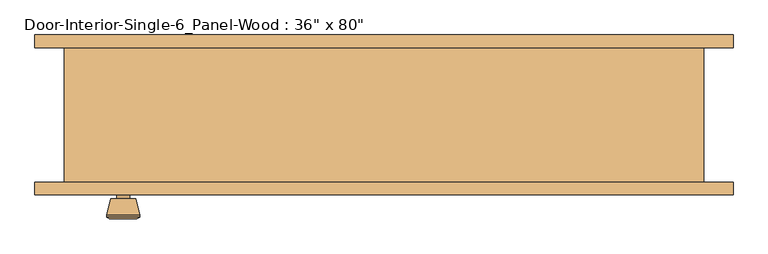
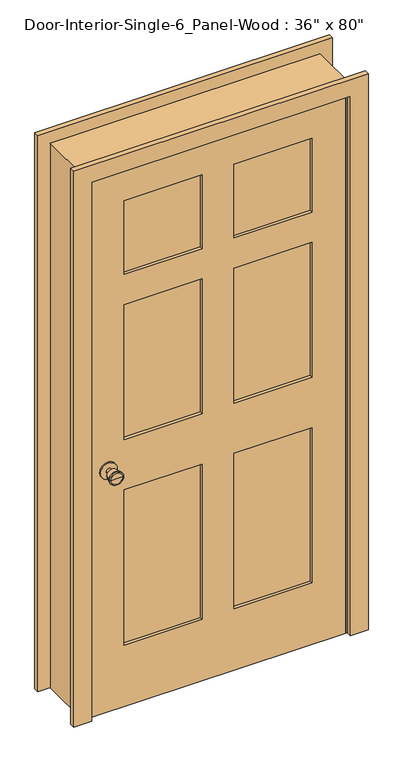
"""IFC4 building model written with IfcOpenShell, lengths in millimetres: door geometry."""

from ifc_helpers import new_model, si_unit, point, frame, frame_2d, origin, place, context, project, spatial, polyline, circle_curve, trimmed, segment, composite_curve, outline, extrude, faceted_brep, source, transform, mapped, element, save
from ifc_brep_helpers import plane_surface, cylinder_surface, revolved_surface, advanced_brep


def door_c2afa946(model_context):
    return source(origin(), model_context, "Body", "SolidModel", [
        advanced_brep(
        [(-393.7, -57.5, 914.4), (-403.7, -57.5, 914.4), (-383.7, -57.5, 914.4), (-373.2241324, -8.5, 914.4), (-414.1758676, -8.5, 914.4), (-393.7, -8.5, 914.4), (-368.7, -10.3278681, 914.4), (-418.7, -10.3278681, 914.4), (-368.7, -13.7915463, 914.4), (-418.7, -13.7915463, 914.4), (-375.063764, -38.5, 914.4), (-412.336236, -38.5, 914.4), (-383.7, -38.5, 914.4), (-403.7, -38.5, 914.4)],
        [
            (0, 1),
            (1, 2, circle_curve(frame((-393.7, -57.5, 914.4), z_axis=(0.0, -1.0, 0.0), x_axis=(-1.0, 0.0, 0.0)), 10.0)),
            (2, 0),
            (2, 1, circle_curve(frame((-393.7, -57.5, 914.4), z_axis=(0.0, -1.0, 0.0), x_axis=(-1.0, 0.0, 0.0)), 10.0)),
            (3, 4, circle_curve(frame((-393.7, -8.5, 914.4), z_axis=(0.0, 1.0, 0.0), x_axis=(-1.0, 0.0, 0.0)), 20.4758676)),
            (4, 5),
            (5, 3),
            (4, 3, circle_curve(frame((-393.7, -8.5, 914.4), z_axis=(0.0, 1.0, 0.0), x_axis=(-1.0, 0.0, 0.0)), 20.4758676)),
            (6, 7, circle_curve(frame((-393.7, -10.3278681, 914.4), z_axis=(0.0, 1.0, 0.0), x_axis=(-1.0, 0.0, 0.0)), 25.0)),
            (7, 4),
            (3, 6),
            (7, 6, circle_curve(frame((-393.7, -10.3278681, 914.4), z_axis=(0.0, 1.0, 0.0), x_axis=(-1.0, 0.0, 0.0)), 25.0)),
            (8, 9, circle_curve(frame((-393.7, -13.7915463, 914.4), z_axis=(0.0, 1.0, 0.0), x_axis=(-1.0, 0.0, 0.0)), 25.0)),
            (9, 7),
            (6, 8),
            (9, 8, circle_curve(frame((-393.7, -13.7915463, 914.4), z_axis=(0.0, 1.0, 0.0), x_axis=(-1.0, 0.0, 0.0)), 25.0)),
            (10, 11, circle_curve(frame((-393.7, -38.5, 914.4), z_axis=(0.0, 1.0, 0.0), x_axis=(-1.0, 0.0, 0.0)), 18.636236)),
            (11, 9),
            (8, 10),
            (11, 10, circle_curve(frame((-393.7, -38.5, 914.4), z_axis=(0.0, 1.0, 0.0), x_axis=(-1.0, 0.0, 0.0)), 18.636236)),
            (12, 13, circle_curve(frame((-393.7, -38.5, 914.4), z_axis=(0.0, 1.0, 0.0), x_axis=(-1.0, 0.0, 0.0)), 10.0)),
            (13, 11),
            (10, 12),
            (13, 12, circle_curve(frame((-393.7, -38.5, 914.4), z_axis=(0.0, 1.0, 0.0), x_axis=(-1.0, 0.0, 0.0)), 10.0)),
            (1, 13),
            (12, 2),
        ],
        [
            plane_surface(frame((-393.7, -57.5, 914.4), z_axis=(0.0, -1.0, 0.0), x_axis=(-1.0, 0.0, 0.0))),
            plane_surface(frame((-393.7, -8.5, 914.4), z_axis=(0.0, 1.0, 0.0), x_axis=(-1.0, 0.0, 0.0))),
            revolved_surface(polyline([(-414.1758676, -8.5, 914.4), (-418.7, -10.3278681, 914.4)]), (-393.7, -57.5, 914.4), (0.0, -1.0, 0.0)),
            cylinder_surface(frame((-393.7, -57.5, 914.4), z_axis=(0.0, -1.0, 0.0), x_axis=(-1.0, 0.0, 0.0)), 25.0),
            revolved_surface(polyline([(-418.7, -13.7915463, 914.4), (-412.336236, -38.5, 914.4)]), (-393.7, -57.5, 914.4), (0.0, -1.0, 0.0)),
            plane_surface(frame((-393.7, -38.5, 914.4), z_axis=(0.0, -1.0, 0.0), x_axis=(-1.0, 0.0, 0.0))),
            cylinder_surface(frame((-393.7, -57.5, 914.4), z_axis=(0.0, -1.0, 0.0), x_axis=(-1.0, 0.0, 0.0)), 10.0),
        ],
        [
            (0, [[1, 2, 3]]),
            (0, [[-3, 4, -1]]),
            (1, [[5, 6, 7]]),
            (1, [[8, -7, -6]]),
            (2, [[9, 10, -5, 11]]),
            (2, [[12, -11, -8, -10]]),
            (3, [[13, 14, -9, 15]]),
            (3, [[16, -15, -12, -14]]),
            (4, [[17, 18, -13, 19]]),
            (4, [[20, -19, -16, -18]]),
            (5, [[21, 22, -17, 23]]),
            (5, [[24, -23, -20, -22]]),
            (6, [[-2, 25, -21, 26]]),
            (6, [[-4, -26, -24, -25]]),
        ],
    ),
        extrude(outline(composite_curve([segment(trimmed(circle_curve(frame_2d((914.4, -393.7)), 30.0), [point((914.4, -423.7))], [point((914.4, -363.7))], False, "CARTESIAN"), True, "CONTINUOUS"), segment(trimmed(circle_curve(frame_2d((914.4, -393.7)), 30.0), [point((914.4, -363.7))], [point((914.4, -423.7))], False, "CARTESIAN"), True, "CONTINUOUS")], self_intersect=False)), frame((0.0, -63.5, 0.0), z_axis=(0.0, 1.0, 0.0), x_axis=(0.0, 0.0, 1.0)), (0.0, 0.0, 1.0), 6.0),
        advanced_brep(
        [(-393.7, -104.425, 914.4), (-383.7, -104.425, 914.4), (-403.7, -104.425, 914.4), (-373.2241324, -153.425, 914.4), (-393.7, -153.425, 914.4), (-414.1758676, -153.425, 914.4), (-368.7, -151.5971319, 914.4), (-418.7, -151.5971319, 914.4), (-368.7, -148.1334537, 914.4), (-418.7, -148.1334537, 914.4), (-375.063764, -123.425, 914.4), (-412.336236, -123.425, 914.4), (-383.7, -123.425, 914.4), (-403.7, -123.425, 914.4)],
        [
            (0, 1),
            (1, 2, circle_curve(frame((-393.7, -104.425, 914.4), z_axis=(0.0, 1.0, 0.0), x_axis=(-1.0, 0.0, 0.0)), 10.0)),
            (2, 0),
            (2, 1, circle_curve(frame((-393.7, -104.425, 914.4), z_axis=(0.0, 1.0, 0.0), x_axis=(-1.0, 0.0, 0.0)), 10.0)),
            (3, 4),
            (4, 5),
            (5, 3, circle_curve(frame((-393.7, -153.425, 914.4), z_axis=(0.0, -1.0, 0.0), x_axis=(-1.0, 0.0, 0.0)), 20.4758676)),
            (3, 5, circle_curve(frame((-393.7, -153.425, 914.4), z_axis=(0.0, -1.0, 0.0), x_axis=(-1.0, 0.0, 0.0)), 20.4758676)),
            (6, 3),
            (5, 7),
            (7, 6, circle_curve(frame((-393.7, -151.5971319, 914.4), z_axis=(0.0, -1.0, 0.0), x_axis=(-1.0, 0.0, 0.0)), 25.0)),
            (6, 7, circle_curve(frame((-393.7, -151.5971319, 914.4), z_axis=(0.0, -1.0, 0.0), x_axis=(-1.0, 0.0, 0.0)), 25.0)),
            (8, 6),
            (7, 9),
            (9, 8, circle_curve(frame((-393.7, -148.1334537, 914.4), z_axis=(0.0, -1.0, 0.0), x_axis=(-1.0, 0.0, 0.0)), 25.0)),
            (8, 9, circle_curve(frame((-393.7, -148.1334537, 914.4), z_axis=(0.0, -1.0, 0.0), x_axis=(-1.0, 0.0, 0.0)), 25.0)),
            (10, 8),
            (9, 11),
            (11, 10, circle_curve(frame((-393.7, -123.425, 914.4), z_axis=(0.0, -1.0, 0.0), x_axis=(-1.0, 0.0, 0.0)), 18.636236)),
            (10, 11, circle_curve(frame((-393.7, -123.425, 914.4), z_axis=(0.0, -1.0, 0.0), x_axis=(-1.0, 0.0, 0.0)), 18.636236)),
            (12, 10),
            (11, 13),
            (13, 12, circle_curve(frame((-393.7, -123.425, 914.4), z_axis=(0.0, -1.0, 0.0), x_axis=(-1.0, 0.0, 0.0)), 10.0)),
            (12, 13, circle_curve(frame((-393.7, -123.425, 914.4), z_axis=(0.0, -1.0, 0.0), x_axis=(-1.0, 0.0, 0.0)), 10.0)),
            (1, 12),
            (13, 2),
        ],
        [
            plane_surface(frame((-393.7, -104.425, 914.4), z_axis=(0.0, 1.0, 0.0), x_axis=(-1.0, 0.0, 0.0))),
            plane_surface(frame((-393.7, -153.425, 914.4), z_axis=(0.0, -1.0, 0.0), x_axis=(-1.0, 0.0, 0.0))),
            revolved_surface(polyline([(-414.1758676, -153.425, 914.4), (-418.7, -151.5971319, 914.4)]), (-393.7, -104.425, 914.4), (0.0, 1.0, 0.0)),
            cylinder_surface(frame((-393.7, -104.425, 914.4), z_axis=(0.0, 1.0, 0.0), x_axis=(-1.0, 0.0, 0.0)), 25.0),
            revolved_surface(polyline([(-418.7, -148.1334537, 914.4), (-412.336236, -123.425, 914.4)]), (-393.7, -104.425, 914.4), (0.0, 1.0, 0.0)),
            plane_surface(frame((-393.7, -123.425, 914.4), z_axis=(0.0, 1.0, 0.0), x_axis=(-1.0, 0.0, 0.0))),
            cylinder_surface(frame((-393.7, -104.425, 914.4), z_axis=(0.0, 1.0, 0.0), x_axis=(-1.0, 0.0, 0.0)), 10.0),
        ],
        [
            (0, [[1, 2, 3]]),
            (0, [[-3, 4, -1]]),
            (1, [[5, 6, 7]]),
            (1, [[-6, -5, 8]]),
            (2, [[9, -7, 10, 11]]),
            (2, [[-10, -8, -9, 12]]),
            (3, [[13, -11, 14, 15]]),
            (3, [[-14, -12, -13, 16]]),
            (4, [[17, -15, 18, 19]]),
            (4, [[-18, -16, -17, 20]]),
            (5, [[21, -19, 22, 23]]),
            (5, [[-22, -20, -21, 24]]),
            (6, [[25, -23, 26, -2]]),
            (6, [[-26, -24, -25, -4]]),
        ],
    ),
        extrude(outline(composite_curve([segment(trimmed(circle_curve(frame_2d((914.4, -393.7)), 30.0), [point((914.4, -423.7))], [point((914.4, -363.7))], False, "CARTESIAN"), True, "CONTINUOUS"), segment(trimmed(circle_curve(frame_2d((914.4, -393.7)), 30.0), [point((914.4, -363.7))], [point((914.4, -423.7))], False, "CARTESIAN"), True, "CONTINUOUS")], self_intersect=False)), frame((0.0, -104.425, 0.0), z_axis=(0.0, 1.0, 0.0), x_axis=(0.0, 0.0, 1.0)), (0.0, 0.0, 1.0), 6.0),
        extrude(outline(polyline([(336.55, -75.1416667), (336.55, -86.7833333), (57.15, -86.7833333), (57.15, -75.1416667), (336.55, -75.1416667)])), frame((0.0, 0.0, 1633.5375), z_axis=(0.0, 0.0, 1.0), x_axis=(1.0, 0.0, 0.0)), (0.0, 0.0, 1.0), 279.4),
        extrude(outline(polyline([(336.55, -75.1416667), (336.55, -86.7833333), (57.15, -86.7833333), (57.15, -75.1416667), (336.55, -75.1416667)])), frame((0.0, 0.0, 1009.65), z_axis=(0.0, 0.0, 1.0), x_axis=(1.0, 0.0, 0.0)), (0.0, 0.0, 1.0), 509.5875),
        extrude(outline(polyline([(-57.15, -75.1416667), (-57.15, -86.7833333), (-336.55, -86.7833333), (-336.55, -75.1416667), (-57.15, -75.1416667)])), frame((0.0, 0.0, 1009.65), z_axis=(0.0, 0.0, 1.0), x_axis=(1.0, 0.0, 0.0)), (0.0, 0.0, 1.0), 509.5875),
        extrude(outline(polyline([(-57.15, -75.1416667), (-57.15, -86.7833333), (-336.55, -86.7833333), (-336.55, -75.1416667), (-57.15, -75.1416667)])), frame((0.0, 0.0, 1633.5375), z_axis=(0.0, 0.0, 1.0), x_axis=(1.0, 0.0, 0.0)), (0.0, 0.0, 1.0), 279.4),
        extrude(outline(polyline([(336.55, -75.1416667), (336.55, -86.7833333), (57.15, -86.7833333), (57.15, -75.1416667), (336.55, -75.1416667)])), frame((0.0, 0.0, 231.775), z_axis=(0.0, 0.0, 1.0), x_axis=(1.0, 0.0, 0.0)), (0.0, 0.0, 1.0), 587.375),
        extrude(outline(polyline([(-57.15, -75.1416667), (-57.15, -86.7833333), (-336.55, -86.7833333), (-336.55, -75.1416667), (-57.15, -75.1416667)])), frame((0.0, 0.0, 231.775), z_axis=(0.0, 0.0, 1.0), x_axis=(1.0, 0.0, 0.0)), (0.0, 0.0, 1.0), 587.375),
        extrude(outline(polyline([(2032.0, -457.2), (0.0, -457.2), (0.0, 457.2), (2032.0, 457.2), (2032.0, -457.2)]), holes=[polyline([(1912.9375, 57.15), (1912.9375, 336.55), (1633.5375, 336.55), (1633.5375, 57.15), (1912.9375, 57.15)]), polyline([(1519.2375, 336.55), (1009.65, 336.55), (1009.65, 57.15), (1519.2375, 57.15), (1519.2375, 336.55)]), polyline([(1009.65, -57.15), (1009.65, -336.55), (1519.2375, -336.55), (1519.2375, -57.15), (1009.65, -57.15)]), polyline([(1633.5375, -336.55), (1912.9375, -336.55), (1912.9375, -57.15), (1633.5375, -57.15), (1633.5375, -336.55)]), polyline([(819.15, 57.15), (819.15, 336.55), (231.775, 336.55), (231.775, 57.15), (819.15, 57.15)]), polyline([(231.775, -57.15), (231.775, -336.55), (819.15, -336.55), (819.15, -57.15), (231.775, -57.15)])]), frame((0.0, -98.425, 0.0), z_axis=(0.0, 1.0, 0.0), x_axis=(0.0, 0.0, 1.0)), (0.0, 0.0, 1.0), 34.925),
        faceted_brep([(482.6, -98.425, 0.0), (457.2, -98.425, 0.0), (457.2, -63.5, 0.0), (444.5, -63.5, 0.0), (444.5, -28.575, 0.0), (457.2, -28.575, 0.0), (457.2, 104.775, 0.0), (482.6, 104.775, 0.0), (482.6, 104.775, 2057.4), (482.6, -98.425, 2057.4), (457.2, 104.775, 2032.0), (-457.2, 104.775, 2032.0), (-457.2, 104.775, 0.0), (-482.6, 104.775, 0.0), (-482.6, 104.775, 2057.4), (457.2, -28.575, 2032.0), (444.5, -28.575, 2019.3), (-444.5, -28.575, 2019.3), (-444.5, -28.575, 0.0), (-457.2, -28.575, 0.0), (-457.2, -28.575, 2032.0), (444.5, -63.5, 2019.3), (457.2, -63.5, 2032.0), (-457.2, -63.5, 2032.0), (-457.2, -63.5, 0.0), (-444.5, -63.5, 0.0), (-444.5, -63.5, 2019.3), (457.2, -98.425, 2032.0), (-482.6, -98.425, 2057.4), (-482.6, -98.425, 0.0), (-457.2, -98.425, 0.0), (-457.2, -98.425, 2032.0)], [[[0, 1, 2, 3, 4, 5, 6, 7]], [[7, 8, 9, 0]], [[6, 10, 11, 12, 13, 14, 8, 7]], [[5, 15, 10, 6]], [[4, 16, 17, 18, 19, 20, 15, 5]], [[3, 21, 16, 4]], [[2, 22, 23, 24, 25, 26, 21, 3]], [[1, 27, 22, 2]], [[0, 9, 28, 29, 30, 31, 27, 1]], [[8, 14, 28, 9]], [[15, 20, 11, 10]], [[21, 26, 17, 16]], [[27, 31, 23, 22]], [[29, 13, 12, 19, 18, 25, 24, 30]], [[14, 13, 29, 28]], [[20, 19, 12, 11]], [[26, 25, 18, 17]], [[31, 30, 24, 23]]]),
        extrude(outline(polyline([(0.0, 527.05), (2101.85, 527.05), (2101.85, -527.05), (0.0, -527.05), (0.0, -463.55), (2038.35, -463.55), (2038.35, 463.55), (0.0, 463.55), (0.0, 527.05)])), frame((0.0, 104.775, 0.0), z_axis=(0.0, 1.0, 0.0), x_axis=(0.0, 0.0, 1.0)), (0.0, 0.0, 1.0), 19.05),
        extrude(outline(polyline([(0.0, 527.05), (2101.85, 527.05), (2101.85, -527.05), (0.0, -527.05), (0.0, -463.55), (2038.35, -463.55), (2038.35, 463.55), (0.0, 463.55), (0.0, 527.05)])), frame((0.0, -117.475, 0.0), z_axis=(0.0, 1.0, 0.0), x_axis=(0.0, 0.0, 1.0)), (0.0, 0.0, 1.0), 19.05),
    ])


if __name__ == "__main__":
    model = new_model("IFC4")
    model_context = context("Model", 3, world=origin())
    ifc_project = project(units=[si_unit("LENGTHUNIT", "METRE", prefix="MILLI")], contexts=[model_context])
    site = spatial("IfcSite", under=ifc_project)
    building = spatial("IfcBuilding", under=site)
    placement = place(None, origin())
    door_shape = door_c2afa946(model_context)
    element("IfcDoor", 1, ObjectType="Door-Interior-Single-6_Panel-Wood : 36\" x 80\"", at=placement, inside=building, context=model_context, shape_type="MappedRepresentation", body=[
        mapped(door_shape, transform((0.0, 0.0, 0.0), x_axis=(1.0, 0.0, 0.0), y_axis=(0.0, 1.0, 0.0), z_axis=(0.0, 0.0, 1.0))),
    ])
    save(model, "model.ifc")

# Revit data of these elements
# Type "Door-Interior-Single-6_Panel-Wood : 36\" x 80\""
#   Type Mark = "9"
#   Assembly Code = "C1020300"
#   Analytic Construction = "Wooden"
#   Top Rail = 0' - 4 11/16"
#   Top Panel = 0' - 11"
#   Thickness = 0' - 1 3/8"
#   Thermal Resistance (R) = 2.5876 (h·ft²·°F)/BTU
#   Swing Angle [instance default] = 90.00°
#   Stiles = 0' - 4 3/4"
#   Rough Width = 3' - 2"
#   Rough Height = 6' - 9"
#   Mullion = 0' - 4 1/2"
#   Lock Rail = 0' - 7 1/2"
#   Intermediate Rail = 0' - 4 1/2"
#   Height = 6' - 8"
#   Width = 3' - 0"
#   Heat Transfer Coefficient (U) = 0.3865 BTU/(h·ft²·°F)
#   Bottom Rail = 0' - 9 1/8"
#   Trim Material = Cherry
#   Panel Material = Cherry
#   Frame Material = Cherry
#   Door Handle Material = Aluminum
#   Visual Light Transmittance = 0
#   Solar Heat Gain Coefficient = 0
#   Wall Closure = (empty or 0)
#   Function = (empty or 0)
# Element 1 (IfcDoor, "Door-Interior-Single-6_Panel-Wood : 36\" x 80\"")
#   Materials on its faces: "Cherry", "Aluminum"
# Materials
#   "Cherry": class "Wood", colour RGB 226 177 128, transparency 0, Description = "Prunus Serotina", Cost = 0
#   "Aluminum": class "Metal", colour RGB 247 247 247, transparency 0, Description = "Aluminum 6061", Cost = 0
